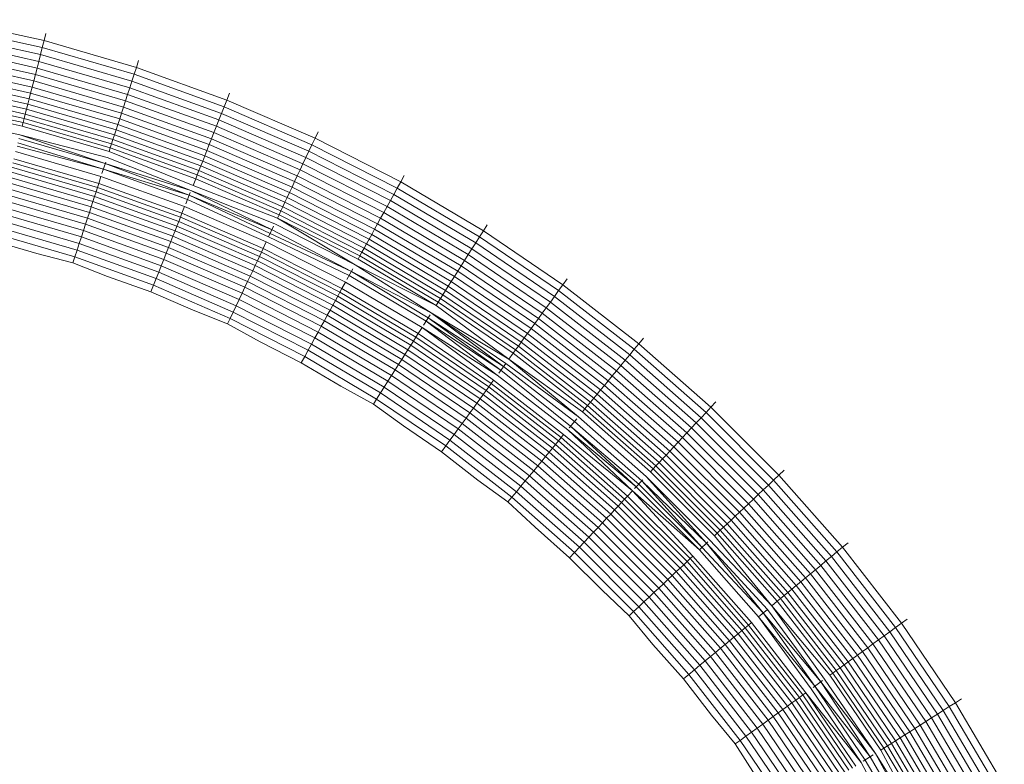
# Model space of a CAD drawing. Units: inches. Extents: x 64 to 1167, y 117 to 939.
# Tile 52 of 56: x 1130.3689 to 1130.6836, y 501.185 to 501.4229. Entities that reach past the tile are written whole.
import ezdxf

# ---------------------------------------------------------------- set-up
doc = ezdxf.new("R2010")
doc.units = ezdxf.units.IN
doc.header["$MEASUREMENT"] = 0
doc.layers.add('A-FLOR-FIXT', color=8, linetype='Continuous', lineweight=18)

msp = doc.modelspace()

# ---------------------------------------------------------------- linework, layer by layer
at = {"layer": 'A-FLOR-FIXT'}
for p, q in [((1130.37673, 501.41624), (1130.34676, 501.42294)), ((1130.37616, 501.41401), (1130.34633, 501.42068)), ((1130.37673, 501.41624), (1130.37731, 501.41848)), ((1130.37504, 501.40963), (1130.34548, 501.41623)), ((1130.3756, 501.41181), (1130.3459, 501.41844)), ((1130.37616, 501.41401), (1130.37673, 501.41624)), ((1130.40623, 501.40767), (1130.37673, 501.41624)), ((1130.37449, 501.40749), (1130.34507, 501.41406)), ((1130.3756, 501.41181), (1130.37616, 501.41401)), ((1130.40552, 501.40549), (1130.37616, 501.41401)), ((1130.37343, 501.40336), (1130.34427, 501.40987)), ((1130.37395, 501.40539), (1130.34466, 501.41194)), ((1130.37449, 501.40749), (1130.37504, 501.40963)), ((1130.37504, 501.40963), (1130.3756, 501.41181)), ((1130.40412, 501.40118), (1130.37504, 501.40963)), ((1130.40481, 501.40332), (1130.3756, 501.41181)), ((1130.40623, 501.40767), (1130.40694, 501.40987)), ((1130.37243, 501.39948), (1130.34352, 501.40595)), ((1130.37292, 501.40138), (1130.34389, 501.40787)), ((1130.37395, 501.40539), (1130.37449, 501.40749)), ((1130.40343, 501.39908), (1130.37449, 501.40749)), ((1130.40552, 501.40549), (1130.40623, 501.40767)), ((1130.43512, 501.39727), (1130.40623, 501.40767)), ((1130.37196, 501.39767), (1130.34317, 501.4041)), ((1130.37292, 501.40138), (1130.37343, 501.40336)), ((1130.37343, 501.40336), (1130.37395, 501.40539)), ((1130.40212, 501.39502), (1130.37343, 501.40336)), ((1130.40277, 501.39702), (1130.37395, 501.40539)), ((1130.40412, 501.40118), (1130.40481, 501.40332)), ((1130.40481, 501.40332), (1130.40552, 501.40549)), ((1130.43344, 501.39301), (1130.40481, 501.40332)), ((1130.43428, 501.39513), (1130.40552, 501.40549)), ((1130.3711, 501.3943), (1130.34252, 501.40069)), ((1130.37152, 501.39594), (1130.34283, 501.40235)), ((1130.37243, 501.39948), (1130.37292, 501.40138)), ((1130.40149, 501.39308), (1130.37292, 501.40138)), ((1130.40343, 501.39908), (1130.40412, 501.40118)), ((1130.43261, 501.39092), (1130.40412, 501.40118)), ((1130.37034, 501.39136), (1130.34195, 501.3977)), ((1130.37071, 501.39278), (1130.34222, 501.39914)), ((1130.37152, 501.39594), (1130.37196, 501.39767)), ((1130.37196, 501.39767), (1130.37243, 501.39948)), ((1130.4003, 501.38943), (1130.37196, 501.39767)), ((1130.40088, 501.39122), (1130.37243, 501.39948)), ((1130.40212, 501.39502), (1130.40277, 501.39702)), ((1130.40277, 501.39702), (1130.40343, 501.39908)), ((1130.431, 501.38686), (1130.40277, 501.39702)), ((1130.4318, 501.38887), (1130.40343, 501.39908)), ((1130.43428, 501.39513), (1130.43512, 501.39727)), ((1130.43512, 501.39727), (1130.43597, 501.39941)), ((1130.46331, 501.38507), (1130.43512, 501.39727)), ((1130.36971, 501.38887), (1130.34147, 501.39518)), ((1130.37001, 501.39005), (1130.34169, 501.39638)), ((1130.37071, 501.39278), (1130.3711, 501.3943)), ((1130.3711, 501.3943), (1130.37152, 501.39594)), ((1130.39923, 501.38613), (1130.3711, 501.3943)), ((1130.39975, 501.38774), (1130.37152, 501.39594)), ((1130.40149, 501.39308), (1130.40212, 501.39502)), ((1130.43023, 501.3849), (1130.40212, 501.39502)), ((1130.43344, 501.39301), (1130.43428, 501.39513)), ((1130.46233, 501.38299), (1130.43428, 501.39513)), ((1130.369, 501.38611), (1130.34093, 501.39238)), ((1130.37001, 501.39005), (1130.37034, 501.39136)), ((1130.37034, 501.39136), (1130.37071, 501.39278)), ((1130.39829, 501.38324), (1130.37034, 501.39136)), ((1130.39874, 501.38463), (1130.37071, 501.39278)), ((1130.4003, 501.38943), (1130.40088, 501.39122)), ((1130.40088, 501.39122), (1130.40149, 501.39308)), ((1130.42876, 501.38118), (1130.40088, 501.39122)), ((1130.42948, 501.38301), (1130.40149, 501.39308)), ((1130.4318, 501.38887), (1130.43261, 501.39092)), ((1130.43261, 501.39092), (1130.43344, 501.39301)), ((1130.4604, 501.37889), (1130.43261, 501.39092)), ((1130.46136, 501.38093), (1130.43344, 501.39301)), ((1130.36971, 501.38887), (1130.37001, 501.39005)), ((1130.3975, 501.3808), (1130.36971, 501.38887)), ((1130.39787, 501.38196), (1130.37001, 501.39005)), ((1130.39923, 501.38613), (1130.39975, 501.38774)), ((1130.39975, 501.38774), (1130.4003, 501.38943)), ((1130.42741, 501.37778), (1130.39975, 501.38774)), ((1130.42806, 501.37944), (1130.4003, 501.38943)), ((1130.431, 501.38686), (1130.4318, 501.38887)), ((1130.45946, 501.37689), (1130.4318, 501.38887)), ((1130.46331, 501.38507), (1130.46429, 501.38716)), ((1130.39624, 501.37695), (1130.3687, 501.38495)), ((1130.39686, 501.37886), (1130.369, 501.38611)), ((1130.39624, 501.37695), (1130.369, 501.38611)), ((1130.39829, 501.38324), (1130.39874, 501.38463)), ((1130.39874, 501.38463), (1130.39923, 501.38613)), ((1130.42621, 501.37474), (1130.39874, 501.38463)), ((1130.42679, 501.37621), (1130.39923, 501.38613)), ((1130.42948, 501.38301), (1130.43023, 501.3849)), ((1130.43023, 501.3849), (1130.431, 501.38686)), ((1130.45765, 501.37304), (1130.43023, 501.3849)), ((1130.45854, 501.37494), (1130.431, 501.38686)), ((1130.46233, 501.38299), (1130.46331, 501.38507)), ((1130.49068, 501.37113), (1130.46331, 501.38507)), ((1130.39491, 501.37284), (1130.36763, 501.38077)), ((1130.39566, 501.37516), (1130.36807, 501.38248)), ((1130.39566, 501.37516), (1130.36836, 501.38364)), ((1130.3975, 501.3808), (1130.39787, 501.38196)), ((1130.42432, 501.36998), (1130.3975, 501.3808)), ((1130.39787, 501.38196), (1130.39829, 501.38324)), ((1130.42517, 501.37213), (1130.39787, 501.38196)), ((1130.42567, 501.37338), (1130.39829, 501.38324)), ((1130.42806, 501.37944), (1130.42876, 501.38118)), ((1130.42876, 501.38118), (1130.42948, 501.38301)), ((1130.45595, 501.36942), (1130.42876, 501.38118)), ((1130.45678, 501.37119), (1130.42948, 501.38301)), ((1130.4604, 501.37889), (1130.46136, 501.38093)), ((1130.46136, 501.38093), (1130.46233, 501.38299)), ((1130.48847, 501.36712), (1130.46136, 501.38093)), ((1130.48957, 501.36911), (1130.46233, 501.38299)), ((1130.3942, 501.37065), (1130.36705, 501.37853)), ((1130.42367, 501.36834), (1130.39686, 501.37886)), ((1130.42679, 501.37621), (1130.42741, 501.37778)), ((1130.42741, 501.37778), (1130.42806, 501.37944)), ((1130.45439, 501.3661), (1130.42741, 501.37778)), ((1130.45515, 501.36772), (1130.42806, 501.37944)), ((1130.45946, 501.37689), (1130.4604, 501.37889)), ((1130.48739, 501.36515), (1130.4604, 501.37889)), ((1130.39333, 501.36797), (1130.36635, 501.37581)), ((1130.39378, 501.36937), (1130.36672, 501.37723)), ((1130.39641, 501.37745), (1130.3952, 501.37375)), ((1130.42254, 501.36548), (1130.39566, 501.37516)), ((1130.42309, 501.36688), (1130.39566, 501.37516)), ((1130.42367, 501.36834), (1130.39624, 501.37695)), ((1130.42309, 501.36688), (1130.39624, 501.37695)), ((1130.42567, 501.37338), (1130.42621, 501.37474)), ((1130.42621, 501.37474), (1130.42679, 501.37621)), ((1130.453, 501.36315), (1130.42621, 501.37474)), ((1130.45367, 501.36458), (1130.42679, 501.37621)), ((1130.45765, 501.37304), (1130.45854, 501.37494)), ((1130.45854, 501.37494), (1130.45946, 501.37689)), ((1130.48528, 501.36131), (1130.45854, 501.37494)), ((1130.48632, 501.36321), (1130.45946, 501.37689)), ((1130.39232, 501.36487), (1130.36554, 501.37265)), ((1130.39284, 501.36647), (1130.36596, 501.37428)), ((1130.39491, 501.37284), (1130.3942, 501.37065)), ((1130.42164, 501.36322), (1130.39491, 501.37284)), ((1130.42432, 501.36998), (1130.42517, 501.37213)), ((1130.42517, 501.37213), (1130.42567, 501.37338)), ((1130.4518, 501.36061), (1130.42517, 501.37213)), ((1130.45237, 501.36182), (1130.42567, 501.37338)), ((1130.45678, 501.37119), (1130.45765, 501.37304)), ((1130.48427, 501.35947), (1130.45765, 501.37304)), ((1130.49068, 501.37113), (1130.49179, 501.37315)), ((1130.39119, 501.36138), (1130.36463, 501.3691)), ((1130.39177, 501.36317), (1130.3651, 501.37092)), ((1130.39378, 501.36937), (1130.39333, 501.36797)), ((1130.3942, 501.37065), (1130.39378, 501.36937)), ((1130.4203, 501.35982), (1130.39378, 501.36937)), ((1130.42079, 501.36107), (1130.3942, 501.37065)), ((1130.45041, 501.35766), (1130.42367, 501.36834)), ((1130.44956, 501.35584), (1130.42367, 501.36834)), ((1130.45128, 501.3595), (1130.42432, 501.36998)), ((1130.45515, 501.36772), (1130.45595, 501.36942)), ((1130.45595, 501.36942), (1130.45678, 501.37119)), ((1130.48234, 501.35597), (1130.45595, 501.36942)), ((1130.48329, 501.35769), (1130.45678, 501.37119)), ((1130.48847, 501.36712), (1130.48957, 501.36911)), ((1130.48957, 501.36911), (1130.49068, 501.37113)), ((1130.51588, 501.35355), (1130.48957, 501.36911)), ((1130.51711, 501.35549), (1130.49068, 501.37113)), ((1130.38995, 501.35758), (1130.36364, 501.36523)), ((1130.39058, 501.35952), (1130.36414, 501.3672)), ((1130.39284, 501.36647), (1130.39232, 501.36487)), ((1130.39333, 501.36797), (1130.39284, 501.36647)), ((1130.41918, 501.35699), (1130.39284, 501.36647)), ((1130.41976, 501.35846), (1130.39333, 501.36797)), ((1130.42342, 501.36772), (1130.42199, 501.3641)), ((1130.44847, 501.35353), (1130.42254, 501.36548)), ((1130.44956, 501.35584), (1130.42309, 501.36688)), ((1130.44898, 501.35461), (1130.42309, 501.36688)), ((1130.45367, 501.36458), (1130.45439, 501.3661)), ((1130.45439, 501.3661), (1130.45515, 501.36772)), ((1130.48058, 501.35276), (1130.45439, 501.3661)), ((1130.48144, 501.35432), (1130.45515, 501.36772)), ((1130.48632, 501.36321), (1130.48739, 501.36515)), ((1130.48739, 501.36515), (1130.48847, 501.36712)), ((1130.51345, 501.34973), (1130.48739, 501.36515)), ((1130.51466, 501.35163), (1130.48847, 501.36712)), ((1130.3893, 501.35558), (1130.36311, 501.36319)), ((1130.39177, 501.36317), (1130.39119, 501.36138)), ((1130.39232, 501.36487), (1130.39177, 501.36317)), ((1130.4179, 501.35376), (1130.39177, 501.36317)), ((1130.41856, 501.35542), (1130.39232, 501.36487)), ((1130.42079, 501.36107), (1130.42164, 501.36322)), ((1130.44772, 501.35193), (1130.42164, 501.36322)), ((1130.45237, 501.36182), (1130.453, 501.36315)), ((1130.453, 501.36315), (1130.45367, 501.36458)), ((1130.47901, 501.3499), (1130.453, 501.36315)), ((1130.47977, 501.35128), (1130.45367, 501.36458)), ((1130.48528, 501.36131), (1130.48632, 501.36321)), ((1130.51227, 501.34786), (1130.48632, 501.36321)), ((1130.38795, 501.35142), (1130.36203, 501.35896)), ((1130.38863, 501.35353), (1130.36258, 501.3611)), ((1130.39058, 501.35952), (1130.38995, 501.35758)), ((1130.39119, 501.36138), (1130.39058, 501.35952)), ((1130.41649, 501.35019), (1130.39058, 501.35952)), ((1130.41721, 501.35202), (1130.39119, 501.36138)), ((1130.41976, 501.35846), (1130.4203, 501.35982)), ((1130.4203, 501.35982), (1130.42079, 501.36107)), ((1130.44616, 501.34863), (1130.4203, 501.35982)), ((1130.44673, 501.34984), (1130.42079, 501.36107)), ((1130.45128, 501.3595), (1130.4518, 501.36061)), ((1130.47608, 501.34458), (1130.45128, 501.3595)), ((1130.47706, 501.34637), (1130.45128, 501.3595)), ((1130.4518, 501.36061), (1130.45237, 501.36182)), ((1130.47765, 501.34744), (1130.4518, 501.36061)), ((1130.4783, 501.34861), (1130.45237, 501.36182)), ((1130.48329, 501.35769), (1130.48427, 501.35947)), ((1130.48427, 501.35947), (1130.48528, 501.36131)), ((1130.50999, 501.34426), (1130.48427, 501.35947)), ((1130.51111, 501.34604), (1130.48528, 501.36131)), ((1130.38726, 501.34929), (1130.36147, 501.35678)), ((1130.3893, 501.35558), (1130.38863, 501.35353)), ((1130.38995, 501.35758), (1130.3893, 501.35558)), ((1130.41496, 501.34634), (1130.3893, 501.35558)), ((1130.41574, 501.3483), (1130.38995, 501.35758)), ((1130.41856, 501.35542), (1130.41918, 501.35699)), ((1130.41918, 501.35699), (1130.41976, 501.35846)), ((1130.44487, 501.34587), (1130.41918, 501.35699)), ((1130.44554, 501.3473), (1130.41976, 501.35846)), ((1130.45006, 501.35692), (1130.44847, 501.35353)), ((1130.47493, 501.34249), (1130.44956, 501.35584)), ((1130.47608, 501.34458), (1130.45041, 501.35766)), ((1130.48144, 501.35432), (1130.48234, 501.35597)), ((1130.48234, 501.35597), (1130.48329, 501.35769)), ((1130.50784, 501.34089), (1130.48234, 501.35597)), ((1130.50889, 501.34254), (1130.48329, 501.35769)), ((1130.51711, 501.35549), (1130.51835, 501.35744)), ((1130.38655, 501.34712), (1130.3609, 501.35457)), ((1130.38863, 501.35353), (1130.38795, 501.35142)), ((1130.41417, 501.34433), (1130.38863, 501.35353)), ((1130.41721, 501.35202), (1130.4179, 501.35376)), ((1130.4179, 501.35376), (1130.41856, 501.35542)), ((1130.44339, 501.34273), (1130.4179, 501.35376)), ((1130.44415, 501.34435), (1130.41856, 501.35542)), ((1130.47421, 501.34117), (1130.44847, 501.35353)), ((1130.47493, 501.34249), (1130.44898, 501.35461)), ((1130.47977, 501.35128), (1130.48058, 501.35276)), ((1130.48058, 501.35276), (1130.48144, 501.35432)), ((1130.50588, 501.33779), (1130.48058, 501.35276)), ((1130.50684, 501.3393), (1130.48144, 501.35432)), ((1130.51466, 501.35163), (1130.51588, 501.35355)), ((1130.51588, 501.35355), (1130.51711, 501.35549)), ((1130.54116, 501.33637), (1130.51588, 501.35355)), ((1130.54251, 501.33823), (1130.51711, 501.35549)), ((1130.37446, 501.34824), (1130.36033, 501.35234)), ((1130.38726, 501.34929), (1130.38655, 501.34712)), ((1130.38795, 501.35142), (1130.38726, 501.34929)), ((1130.41252, 501.34019), (1130.38726, 501.34929)), ((1130.41335, 501.34228), (1130.38795, 501.35142)), ((1130.41574, 501.3483), (1130.41649, 501.35019)), ((1130.41649, 501.35019), (1130.41721, 501.35202)), ((1130.44175, 501.33926), (1130.41649, 501.35019)), ((1130.44259, 501.34103), (1130.41721, 501.35202)), ((1130.44616, 501.34863), (1130.44673, 501.34984)), ((1130.44673, 501.34984), (1130.44772, 501.35193)), ((1130.47192, 501.33701), (1130.44673, 501.34984)), ((1130.47303, 501.33903), (1130.44772, 501.35193)), ((1130.47901, 501.3499), (1130.4783, 501.34861)), ((1130.47977, 501.35128), (1130.47901, 501.3499)), ((1130.50413, 501.33504), (1130.47901, 501.3499)), ((1130.50498, 501.33637), (1130.47977, 501.35128)), ((1130.51227, 501.34786), (1130.51345, 501.34973)), ((1130.51345, 501.34973), (1130.51466, 501.35163)), ((1130.5385, 501.33271), (1130.51345, 501.34973)), ((1130.53982, 501.33453), (1130.51466, 501.35163)), ((1130.38596, 501.34529), (1130.37446, 501.34824)), ((1130.38655, 501.34712), (1130.38596, 501.34529)), ((1130.41169, 501.33807), (1130.38655, 501.34712)), ((1130.41417, 501.34433), (1130.41496, 501.34634)), ((1130.41496, 501.34634), (1130.41574, 501.3483)), ((1130.43999, 501.33551), (1130.41496, 501.34634)), ((1130.44089, 501.33742), (1130.41574, 501.3483)), ((1130.44487, 501.34587), (1130.44554, 501.3473)), ((1130.44554, 501.3473), (1130.44616, 501.34863)), ((1130.47057, 501.33455), (1130.44554, 501.3473)), ((1130.47127, 501.33583), (1130.44616, 501.34863)), ((1130.47765, 501.34744), (1130.47706, 501.34637)), ((1130.50197, 501.33164), (1130.47706, 501.34637)), ((1130.4783, 501.34861), (1130.47765, 501.34744)), ((1130.50263, 501.33267), (1130.47765, 501.34744)), ((1130.50335, 501.3338), (1130.4783, 501.34861)), ((1130.51111, 501.34604), (1130.51227, 501.34786)), ((1130.5372, 501.33092), (1130.51227, 501.34786)), ((1130.397, 501.34092), (1130.38596, 501.34529)), ((1130.41335, 501.34228), (1130.41417, 501.34433)), ((1130.43907, 501.33356), (1130.41417, 501.34433)), ((1130.44339, 501.34273), (1130.44415, 501.34435)), ((1130.44415, 501.34435), (1130.44487, 501.34587)), ((1130.46899, 501.33169), (1130.44415, 501.34435)), ((1130.46981, 501.33316), (1130.44487, 501.34587)), ((1130.47537, 501.34328), (1130.47349, 501.33987)), ((1130.50044, 501.32922), (1130.47608, 501.34458)), ((1130.50197, 501.33164), (1130.47608, 501.34458)), ((1130.50889, 501.34254), (1130.50999, 501.34426)), ((1130.50999, 501.34426), (1130.51111, 501.34604)), ((1130.5347, 501.32747), (1130.50999, 501.34426)), ((1130.53593, 501.32917), (1130.51111, 501.34604)), ((1130.41084, 501.33593), (1130.397, 501.34092)), ((1130.41169, 501.33807), (1130.41252, 501.34019)), ((1130.41252, 501.34019), (1130.41335, 501.34228)), ((1130.43717, 501.32952), (1130.41252, 501.34019)), ((1130.43813, 501.33156), (1130.41335, 501.34228)), ((1130.44175, 501.33926), (1130.44259, 501.34103)), ((1130.44259, 501.34103), (1130.44339, 501.34273)), ((1130.46723, 501.32848), (1130.44259, 501.34103)), ((1130.46813, 501.33012), (1130.44339, 501.34273)), ((1130.49879, 501.32663), (1130.47421, 501.34117)), ((1130.50044, 501.32922), (1130.47493, 501.34249)), ((1130.49948, 501.32771), (1130.47493, 501.34249)), ((1130.50684, 501.3393), (1130.50784, 501.34089)), ((1130.50784, 501.34089), (1130.50889, 501.34254)), ((1130.53235, 501.32423), (1130.50784, 501.34089)), ((1130.5335, 501.32582), (1130.50889, 501.34254)), ((1130.54251, 501.33823), (1130.54387, 501.3401)), ((1130.41084, 501.33593), (1130.41169, 501.33807)), ((1130.4362, 501.32746), (1130.41169, 501.33807)), ((1130.43999, 501.33551), (1130.44089, 501.33742)), ((1130.44089, 501.33742), (1130.44175, 501.33926)), ((1130.4653, 501.32497), (1130.44089, 501.33742)), ((1130.46629, 501.32676), (1130.44175, 501.33926)), ((1130.47192, 501.33701), (1130.47127, 501.33583)), ((1130.47192, 501.33701), (1130.47303, 501.33903)), ((1130.49625, 501.32262), (1130.47192, 501.33701)), ((1130.49749, 501.32457), (1130.47303, 501.33903)), ((1130.50498, 501.33637), (1130.50588, 501.33779)), ((1130.50588, 501.33779), (1130.50684, 501.3393)), ((1130.53019, 501.32127), (1130.50588, 501.33779)), ((1130.53124, 501.32272), (1130.50684, 501.3393)), ((1130.54116, 501.33637), (1130.54251, 501.33823)), ((1130.56678, 501.31941), (1130.54251, 501.33823)), ((1130.42434, 501.33009), (1130.41084, 501.33593)), ((1130.43813, 501.33156), (1130.43907, 501.33356)), ((1130.43907, 501.33356), (1130.43999, 501.33551)), ((1130.46325, 501.32124), (1130.43907, 501.33356)), ((1130.46429, 501.32313), (1130.43999, 501.33551)), ((1130.47057, 501.33455), (1130.46981, 501.33316)), ((1130.47127, 501.33583), (1130.47057, 501.33455)), ((1130.49475, 501.32025), (1130.47057, 501.33455)), ((1130.49553, 501.32149), (1130.47127, 501.33583)), ((1130.50263, 501.33267), (1130.50335, 501.3338)), ((1130.50335, 501.3338), (1130.50413, 501.33504)), ((1130.52741, 501.31745), (1130.50335, 501.3338)), ((1130.50413, 501.33504), (1130.50498, 501.33637)), ((1130.52828, 501.31863), (1130.50413, 501.33504)), ((1130.5292, 501.31991), (1130.50498, 501.33637)), ((1130.5385, 501.33271), (1130.53982, 501.33453)), ((1130.53982, 501.33453), (1130.54116, 501.33637)), ((1130.56387, 501.31588), (1130.53982, 501.33453)), ((1130.56532, 501.31763), (1130.54116, 501.33637)), ((1130.43717, 501.32952), (1130.43813, 501.33156)), ((1130.46218, 501.3193), (1130.43813, 501.33156)), ((1130.46899, 501.33169), (1130.46813, 501.33012)), ((1130.46981, 501.33316), (1130.46899, 501.33169)), ((1130.493, 501.31749), (1130.46899, 501.33169)), ((1130.4939, 501.31892), (1130.46981, 501.33316)), ((1130.50197, 501.33164), (1130.50263, 501.33267)), ((1130.52527, 501.31449), (1130.50197, 501.33164)), ((1130.52662, 501.31636), (1130.50263, 501.33267)), ((1130.53593, 501.32917), (1130.5372, 501.33092)), ((1130.5372, 501.33092), (1130.5385, 501.33271)), ((1130.56102, 501.31244), (1130.5372, 501.33092)), ((1130.56243, 501.31415), (1130.5385, 501.33271)), ((1130.43538, 501.32572), (1130.42434, 501.33009)), ((1130.43538, 501.32572), (1130.4362, 501.32746)), ((1130.4362, 501.32746), (1130.43717, 501.32952)), ((1130.46, 501.31533), (1130.4362, 501.32746)), ((1130.4611, 501.31733), (1130.43717, 501.32952)), ((1130.46723, 501.32848), (1130.46629, 501.32676)), ((1130.46813, 501.33012), (1130.46723, 501.32848)), ((1130.49103, 501.3144), (1130.46723, 501.32848)), ((1130.49204, 501.31599), (1130.46813, 501.33012)), ((1130.50008, 501.32866), (1130.498, 501.32538)), ((1130.52353, 501.31209), (1130.49948, 501.32771)), ((1130.52273, 501.311), (1130.49948, 501.32771)), ((1130.52527, 501.31449), (1130.50044, 501.32922)), ((1130.52423, 501.31306), (1130.50044, 501.32922)), ((1130.52353, 501.31209), (1130.50044, 501.32922)), ((1130.5335, 501.32582), (1130.5347, 501.32747)), ((1130.5347, 501.32747), (1130.53593, 501.32917)), ((1130.5583, 501.30916), (1130.5347, 501.32747)), ((1130.55965, 501.31078), (1130.53593, 501.32917)), ((1130.44579, 501.32), (1130.43538, 501.32572)), ((1130.4653, 501.32497), (1130.46429, 501.32313)), ((1130.46629, 501.32676), (1130.4653, 501.32497)), ((1130.48889, 501.31102), (1130.4653, 501.32497)), ((1130.48998, 501.31274), (1130.46629, 501.32676)), ((1130.49749, 501.32457), (1130.49625, 501.32262)), ((1130.52035, 501.30772), (1130.49749, 501.32457)), ((1130.52155, 501.30937), (1130.49749, 501.32457)), ((1130.52273, 501.311), (1130.49879, 501.32663)), ((1130.52155, 501.30937), (1130.49879, 501.32663)), ((1130.53124, 501.32272), (1130.53235, 501.32423)), ((1130.53235, 501.32423), (1130.5335, 501.32582)), ((1130.55576, 501.30608), (1130.53235, 501.32423)), ((1130.55701, 501.30759), (1130.5335, 501.32582)), ((1130.46325, 501.32124), (1130.46218, 501.3193)), ((1130.46429, 501.32313), (1130.46325, 501.32124)), ((1130.48661, 501.30742), (1130.46325, 501.32124)), ((1130.48777, 501.30925), (1130.46429, 501.32313)), ((1130.49475, 501.32025), (1130.49553, 501.32149)), ((1130.49553, 501.32149), (1130.49625, 501.32262)), ((1130.51884, 501.30564), (1130.49553, 501.32149)), ((1130.51963, 501.30673), (1130.49625, 501.32262)), ((1130.5292, 501.31991), (1130.53019, 501.32127)), ((1130.53019, 501.32127), (1130.53124, 501.32272)), ((1130.55342, 501.30325), (1130.53019, 501.32127)), ((1130.55456, 501.30463), (1130.53124, 501.32272)), ((1130.56678, 501.31941), (1130.56825, 501.32118)), ((1130.4589, 501.31332), (1130.44579, 501.32)), ((1130.46218, 501.3193), (1130.4611, 501.31733)), ((1130.48542, 501.30556), (1130.46218, 501.3193)), ((1130.493, 501.31749), (1130.4939, 501.31892)), ((1130.4939, 501.31892), (1130.49475, 501.32025)), ((1130.51705, 501.30318), (1130.4939, 501.31892)), ((1130.51798, 501.30446), (1130.49475, 501.32025)), ((1130.52741, 501.31745), (1130.52828, 501.31863)), ((1130.52828, 501.31863), (1130.5292, 501.31991)), ((1130.55134, 501.30074), (1130.52828, 501.31863)), ((1130.55235, 501.30196), (1130.5292, 501.31991)), ((1130.56532, 501.31763), (1130.56678, 501.31941)), ((1130.58982, 501.29909), (1130.56678, 501.31941)), ((1130.46, 501.31533), (1130.4589, 501.31332)), ((1130.4611, 501.31733), (1130.46, 501.31533)), ((1130.483, 501.30173), (1130.46, 501.31533)), ((1130.48422, 501.30366), (1130.4611, 501.31733)), ((1130.49103, 501.3144), (1130.49204, 501.31599)), ((1130.49204, 501.31599), (1130.493, 501.31749)), ((1130.51501, 501.30037), (1130.49204, 501.31599)), ((1130.51606, 501.30182), (1130.493, 501.31749)), ((1130.52527, 501.31449), (1130.52662, 501.31636)), ((1130.52662, 501.31636), (1130.52741, 501.31745)), ((1130.54955, 501.29857), (1130.52662, 501.31636)), ((1130.55041, 501.29961), (1130.52741, 501.31745)), ((1130.56243, 501.31415), (1130.56387, 501.31588)), ((1130.56387, 501.31588), (1130.56532, 501.31763)), ((1130.58669, 501.29576), (1130.56387, 501.31588)), ((1130.58825, 501.29742), (1130.56532, 501.31763)), ((1130.47156, 501.30583), (1130.4589, 501.31332)), ((1130.48889, 501.31102), (1130.48998, 501.31274)), ((1130.48998, 501.31274), (1130.49103, 501.3144)), ((1130.51276, 501.29727), (1130.48998, 501.31274)), ((1130.51391, 501.29886), (1130.49103, 501.3144)), ((1130.52423, 501.31306), (1130.52203, 501.31003)), ((1130.54619, 501.29451), (1130.52353, 501.31209)), ((1130.54747, 501.29606), (1130.52423, 501.31306)), ((1130.54877, 501.29763), (1130.52527, 501.31449)), ((1130.54747, 501.29606), (1130.52527, 501.31449)), ((1130.55965, 501.31078), (1130.56102, 501.31244)), ((1130.56102, 501.31244), (1130.56243, 501.31415)), ((1130.58364, 501.29251), (1130.56102, 501.31244)), ((1130.58515, 501.29412), (1130.56243, 501.31415)), ((1130.48661, 501.30742), (1130.48777, 501.30925)), ((1130.48777, 501.30925), (1130.48889, 501.31102)), ((1130.51032, 501.29392), (1130.48777, 501.30925)), ((1130.51156, 501.29562), (1130.48889, 501.31102)), ((1130.54405, 501.29192), (1130.52155, 501.30937)), ((1130.54499, 501.29306), (1130.52273, 501.311)), ((1130.55701, 501.30759), (1130.5583, 501.30916)), ((1130.5583, 501.30916), (1130.55965, 501.31078)), ((1130.58072, 501.2894), (1130.5583, 501.30916)), ((1130.58216, 501.29093), (1130.55965, 501.31078)), ((1130.48197, 501.30011), (1130.47156, 501.30583)), ((1130.48422, 501.30366), (1130.48542, 501.30556)), ((1130.48542, 501.30556), (1130.48661, 501.30742)), ((1130.50775, 501.29038), (1130.48542, 501.30556)), ((1130.50905, 501.29217), (1130.48661, 501.30742)), ((1130.51798, 501.30446), (1130.51884, 501.30564)), ((1130.51884, 501.30564), (1130.51963, 501.30673)), ((1130.54111, 501.28837), (1130.51884, 501.30564)), ((1130.51963, 501.30673), (1130.52035, 501.30772)), ((1130.54197, 501.28941), (1130.51963, 501.30673)), ((1130.54274, 501.29035), (1130.52035, 501.30772)), ((1130.55456, 501.30463), (1130.55576, 501.30608)), ((1130.55576, 501.30608), (1130.55701, 501.30759)), ((1130.57798, 501.28648), (1130.55576, 501.30608)), ((1130.57932, 501.28791), (1130.55701, 501.30759)), ((1130.483, 501.30173), (1130.48422, 501.30366)), ((1130.50643, 501.28856), (1130.48422, 501.30366)), ((1130.51606, 501.30182), (1130.51705, 501.30318)), ((1130.51705, 501.30318), (1130.51798, 501.30446)), ((1130.53917, 501.28603), (1130.51705, 501.30318)), ((1130.54018, 501.28724), (1130.51798, 501.30446)), ((1130.55235, 501.30196), (1130.55342, 501.30325)), ((1130.55342, 501.30325), (1130.55456, 501.30463)), ((1130.57547, 501.28381), (1130.55342, 501.30325)), ((1130.57669, 501.28512), (1130.55456, 501.30463)), ((1130.48197, 501.30011), (1130.483, 501.30173)), ((1130.49157, 501.29313), (1130.48197, 501.30011)), ((1130.50509, 501.28672), (1130.483, 501.30173)), ((1130.51391, 501.29886), (1130.51501, 501.30037)), ((1130.51501, 501.30037), (1130.51606, 501.30182)), ((1130.53696, 501.28335), (1130.51501, 501.30037)), ((1130.53809, 501.28473), (1130.51606, 501.30182)), ((1130.54955, 501.29857), (1130.55041, 501.29961)), ((1130.55041, 501.29961), (1130.55134, 501.30074)), ((1130.57223, 501.28037), (1130.55041, 501.29961)), ((1130.55134, 501.30074), (1130.55235, 501.30196)), ((1130.57324, 501.28143), (1130.55134, 501.30074)), ((1130.57432, 501.28259), (1130.55235, 501.30196)), ((1130.58825, 501.29742), (1130.58982, 501.29909)), ((1130.58982, 501.29909), (1130.5914, 501.30078)), ((1130.61154, 501.27738), (1130.58982, 501.29909)), ((1130.51156, 501.29562), (1130.51276, 501.29727)), ((1130.51276, 501.29727), (1130.51391, 501.29886)), ((1130.53451, 501.28039), (1130.51276, 501.29727)), ((1130.53576, 501.28191), (1130.51391, 501.29886)), ((1130.56908, 501.27701), (1130.54747, 501.29606)), ((1130.54877, 501.29763), (1130.54955, 501.29857)), ((1130.57048, 501.2785), (1130.54877, 501.29763)), ((1130.57131, 501.27939), (1130.54955, 501.29857)), ((1130.58669, 501.29576), (1130.58825, 501.29742)), ((1130.60986, 501.2758), (1130.58825, 501.29742)), ((1130.50374, 501.28486), (1130.49157, 501.29313)), ((1130.50905, 501.29217), (1130.51032, 501.29392)), ((1130.51032, 501.29392), (1130.51156, 501.29562)), ((1130.53187, 501.2772), (1130.51032, 501.29392)), ((1130.53321, 501.27882), (1130.51156, 501.29562)), ((1130.54695, 501.29543), (1130.54456, 501.29255)), ((1130.56596, 501.27369), (1130.54499, 501.29306)), ((1130.56678, 501.27456), (1130.54499, 501.29306)), ((1130.56771, 501.27554), (1130.54619, 501.29451)), ((1130.58364, 501.29251), (1130.58515, 501.29412)), ((1130.58515, 501.29412), (1130.58669, 501.29576)), ((1130.60656, 501.2727), (1130.58515, 501.29412)), ((1130.6082, 501.27424), (1130.58669, 501.29576)), ((1130.50643, 501.28856), (1130.50775, 501.29038)), ((1130.50775, 501.29038), (1130.50905, 501.29217)), ((1130.52908, 501.27384), (1130.50775, 501.29038)), ((1130.53049, 501.27554), (1130.50905, 501.29217)), ((1130.54197, 501.28941), (1130.54274, 501.29035)), ((1130.56475, 501.2724), (1130.54274, 501.29035)), ((1130.56475, 501.2724), (1130.54405, 501.29192)), ((1130.56596, 501.27369), (1130.54405, 501.29192)), ((1130.58072, 501.2894), (1130.58216, 501.29093)), ((1130.58216, 501.29093), (1130.58364, 501.29251)), ((1130.60338, 501.26971), (1130.58216, 501.29093)), ((1130.60495, 501.27119), (1130.58364, 501.29251)), ((1130.50374, 501.28486), (1130.50509, 501.28672)), ((1130.50509, 501.28672), (1130.50643, 501.28856)), ((1130.5262, 501.27035), (1130.50509, 501.28672)), ((1130.52765, 501.2721), (1130.50643, 501.28856)), ((1130.53917, 501.28603), (1130.54018, 501.28724)), ((1130.54018, 501.28724), (1130.54111, 501.28837)), ((1130.56125, 501.26867), (1130.54018, 501.28724)), ((1130.54111, 501.28837), (1130.54197, 501.28941)), ((1130.56225, 501.26973), (1130.54111, 501.28837)), ((1130.56317, 501.27071), (1130.54197, 501.28941)), ((1130.57669, 501.28512), (1130.57798, 501.28648)), ((1130.57798, 501.28648), (1130.57932, 501.28791)), ((1130.59893, 501.26554), (1130.57798, 501.28648)), ((1130.57932, 501.28791), (1130.58072, 501.2894)), ((1130.60036, 501.26688), (1130.57932, 501.28791)), ((1130.60184, 501.26827), (1130.58072, 501.2894)), ((1130.51537, 501.27584), (1130.50374, 501.28486)), ((1130.53576, 501.28191), (1130.53696, 501.28335)), ((1130.53696, 501.28335), (1130.53809, 501.28473)), ((1130.55779, 501.26499), (1130.53696, 501.28335)), ((1130.53809, 501.28473), (1130.53917, 501.28603)), ((1130.55901, 501.26629), (1130.53809, 501.28473)), ((1130.56017, 501.26752), (1130.53917, 501.28603)), ((1130.57432, 501.28259), (1130.57547, 501.28381)), ((1130.57547, 501.28381), (1130.57669, 501.28512)), ((1130.59626, 501.26303), (1130.57547, 501.28381)), ((1130.59756, 501.26425), (1130.57669, 501.28512)), ((1130.53321, 501.27882), (1130.53451, 501.28039)), ((1130.53451, 501.28039), (1130.53576, 501.28191)), ((1130.55516, 501.26219), (1130.53451, 501.28039)), ((1130.5565, 501.26362), (1130.53576, 501.28191)), ((1130.57131, 501.27939), (1130.57223, 501.28037)), ((1130.57223, 501.28037), (1130.57324, 501.28143)), ((1130.59281, 501.25979), (1130.57223, 501.28037)), ((1130.57324, 501.28143), (1130.57432, 501.28259)), ((1130.59388, 501.26079), (1130.57324, 501.28143)), ((1130.59503, 501.26187), (1130.57432, 501.28259)), ((1130.53049, 501.27554), (1130.53187, 501.2772)), ((1130.53187, 501.2772), (1130.53321, 501.27882)), ((1130.55233, 501.25917), (1130.53187, 501.2772)), ((1130.55377, 501.2607), (1130.53321, 501.27882)), ((1130.58837, 501.25562), (1130.56908, 501.27701)), ((1130.58945, 501.25664), (1130.56908, 501.27701)), ((1130.57048, 501.2785), (1130.57131, 501.27939)), ((1130.59094, 501.25803), (1130.57048, 501.2785)), ((1130.59183, 501.25887), (1130.57131, 501.27939)), ((1130.61154, 501.27738), (1130.60986, 501.2758)), ((1130.61322, 501.27896), (1130.61154, 501.27738)), ((1130.63185, 501.25434), (1130.61154, 501.27738)), ((1130.52497, 501.26886), (1130.51537, 501.27584)), ((1130.52765, 501.2721), (1130.52908, 501.27384)), ((1130.52908, 501.27384), (1130.53049, 501.27554)), ((1130.54934, 501.25598), (1130.52908, 501.27384)), ((1130.55085, 501.25759), (1130.53049, 501.27554)), ((1130.56806, 501.27593), (1130.5654, 501.27309)), ((1130.587, 501.25433), (1130.56678, 501.27456)), ((1130.58837, 501.25562), (1130.56771, 501.27554)), ((1130.587, 501.25433), (1130.56771, 501.27554)), ((1130.6082, 501.27424), (1130.60656, 501.2727)), ((1130.60986, 501.2758), (1130.6082, 501.27424)), ((1130.62832, 501.25142), (1130.6082, 501.27424)), ((1130.63008, 501.25287), (1130.60986, 501.2758)), ((1130.5262, 501.27035), (1130.52765, 501.2721)), ((1130.5478, 501.25434), (1130.52765, 501.2721)), ((1130.56225, 501.26973), (1130.56317, 501.27071)), ((1130.56317, 501.27071), (1130.56475, 501.2724)), ((1130.58316, 501.25073), (1130.56317, 501.27071)), ((1130.58405, 501.25156), (1130.56475, 501.2724)), ((1130.58613, 501.25352), (1130.56475, 501.2724)), ((1130.58613, 501.25352), (1130.56596, 501.27369)), ((1130.60495, 501.27119), (1130.60338, 501.26971)), ((1130.60656, 501.2727), (1130.60495, 501.27119)), ((1130.62489, 501.24858), (1130.60495, 501.27119)), ((1130.62659, 501.24999), (1130.60656, 501.2727)), ((1130.52497, 501.26886), (1130.5262, 501.27035)), ((1130.53363, 501.26074), (1130.52497, 501.26886)), ((1130.54624, 501.25268), (1130.5262, 501.27035)), ((1130.55901, 501.26629), (1130.56017, 501.26752)), ((1130.56017, 501.26752), (1130.56125, 501.26867)), ((1130.57996, 501.24772), (1130.56017, 501.26752)), ((1130.56125, 501.26867), (1130.56225, 501.26973)), ((1130.58111, 501.2488), (1130.56125, 501.26867)), ((1130.58218, 501.24981), (1130.56225, 501.26973)), ((1130.60184, 501.26827), (1130.60036, 501.26688)), ((1130.60338, 501.26971), (1130.60184, 501.26827)), ((1130.6216, 501.24586), (1130.60184, 501.26827)), ((1130.62322, 501.2472), (1130.60338, 501.26971)), ((1130.5565, 501.26362), (1130.55779, 501.26499)), ((1130.55779, 501.26499), (1130.55901, 501.26629)), ((1130.57743, 501.24535), (1130.55779, 501.26499)), ((1130.57873, 501.24657), (1130.55901, 501.26629)), ((1130.59893, 501.26554), (1130.59756, 501.26425)), ((1130.60036, 501.26688), (1130.59893, 501.26554)), ((1130.61852, 501.24331), (1130.59893, 501.26554)), ((1130.62003, 501.24456), (1130.60036, 501.26688)), ((1130.55377, 501.2607), (1130.55516, 501.26219)), ((1130.55516, 501.26219), (1130.5565, 501.26362)), ((1130.57463, 501.24272), (1130.55516, 501.26219)), ((1130.57606, 501.24406), (1130.5565, 501.26362)), ((1130.59503, 501.26187), (1130.59388, 501.26079)), ((1130.59626, 501.26303), (1130.59503, 501.26187)), ((1130.6144, 501.2399), (1130.59503, 501.26187)), ((1130.59756, 501.26425), (1130.59626, 501.26303)), ((1130.6157, 501.24098), (1130.59626, 501.26303)), ((1130.61707, 501.24212), (1130.59756, 501.26425)), ((1130.54466, 501.25101), (1130.53363, 501.26074)), ((1130.55085, 501.25759), (1130.55233, 501.25917)), ((1130.55233, 501.25917), (1130.55377, 501.2607)), ((1130.57161, 501.23988), (1130.55233, 501.25917)), ((1130.57315, 501.24132), (1130.55377, 501.2607)), ((1130.59183, 501.25887), (1130.59094, 501.25803)), ((1130.60924, 501.23563), (1130.59094, 501.25803)), ((1130.59281, 501.25979), (1130.59183, 501.25887)), ((1130.61102, 501.23711), (1130.59183, 501.25887)), ((1130.59388, 501.26079), (1130.59281, 501.25979)), ((1130.61205, 501.23796), (1130.59281, 501.25979)), ((1130.61318, 501.2389), (1130.59388, 501.26079)), ((1130.5478, 501.25434), (1130.54934, 501.25598)), ((1130.54934, 501.25598), (1130.55085, 501.25759)), ((1130.56843, 501.23689), (1130.54934, 501.25598)), ((1130.57004, 501.2384), (1130.55085, 501.25759)), ((1130.58886, 501.25608), (1130.58613, 501.25352)), ((1130.60649, 501.23336), (1130.58837, 501.25562)), ((1130.60788, 501.23451), (1130.58837, 501.25562)), ((1130.60924, 501.23563), (1130.58945, 501.25664)), ((1130.63185, 501.25434), (1130.63363, 501.25581)), ((1130.54466, 501.25101), (1130.54624, 501.25268)), ((1130.54624, 501.25268), (1130.5478, 501.25434)), ((1130.56512, 501.23379), (1130.54624, 501.25268)), ((1130.56679, 501.23535), (1130.5478, 501.25434)), ((1130.60499, 501.23212), (1130.58613, 501.25352)), ((1130.60649, 501.23336), (1130.587, 501.25433)), ((1130.62832, 501.25142), (1130.63008, 501.25287)), ((1130.63008, 501.25287), (1130.63185, 501.25434)), ((1130.64881, 501.22872), (1130.63008, 501.25287)), ((1130.65067, 501.23007), (1130.63185, 501.25434)), ((1130.55507, 501.2406), (1130.54466, 501.25101)), ((1130.57996, 501.24772), (1130.58111, 501.2488)), ((1130.58111, 501.2488), (1130.58218, 501.24981)), ((1130.59969, 501.22773), (1130.58111, 501.2488)), ((1130.58218, 501.24981), (1130.58316, 501.25073)), ((1130.60081, 501.22867), (1130.58218, 501.24981)), ((1130.58316, 501.25073), (1130.58405, 501.25156)), ((1130.60185, 501.22952), (1130.58316, 501.25073)), ((1130.60279, 501.2303), (1130.58405, 501.25156)), ((1130.62322, 501.2472), (1130.62489, 501.24858)), ((1130.62489, 501.24858), (1130.62659, 501.24999)), ((1130.64336, 501.22476), (1130.62489, 501.24858)), ((1130.62659, 501.24999), (1130.62832, 501.25142)), ((1130.64515, 501.22606), (1130.62659, 501.24999)), ((1130.64697, 501.22738), (1130.62832, 501.25142)), ((1130.57743, 501.24535), (1130.57873, 501.24657)), ((1130.57873, 501.24657), (1130.57996, 501.24772)), ((1130.59717, 501.22565), (1130.57873, 501.24657)), ((1130.59847, 501.22673), (1130.57996, 501.24772)), ((1130.62003, 501.24456), (1130.6216, 501.24586)), ((1130.6216, 501.24586), (1130.62322, 501.2472)), ((1130.63991, 501.22225), (1130.6216, 501.24586)), ((1130.64161, 501.22349), (1130.62322, 501.2472)), ((1130.57315, 501.24132), (1130.57463, 501.24272)), ((1130.57463, 501.24272), (1130.57606, 501.24406)), ((1130.59284, 501.22207), (1130.57463, 501.24272)), ((1130.57606, 501.24406), (1130.57743, 501.24535)), ((1130.59435, 501.22332), (1130.57606, 501.24406)), ((1130.5958, 501.22451), (1130.57743, 501.24535)), ((1130.61707, 501.24212), (1130.61852, 501.24331)), ((1130.61852, 501.24331), (1130.62003, 501.24456)), ((1130.63668, 501.2199), (1130.61852, 501.24331)), ((1130.63826, 501.22106), (1130.62003, 501.24456)), ((1130.56372, 501.23247), (1130.55507, 501.2406)), ((1130.57004, 501.2384), (1130.57161, 501.23988)), ((1130.57315, 501.24132), (1130.57161, 501.23988)), ((1130.58965, 501.21943), (1130.57161, 501.23988)), ((1130.59127, 501.22077), (1130.57315, 501.24132)), ((1130.61318, 501.2389), (1130.6144, 501.2399)), ((1130.6144, 501.2399), (1130.6157, 501.24098)), ((1130.63235, 501.21676), (1130.6144, 501.2399)), ((1130.6157, 501.24098), (1130.61707, 501.24212)), ((1130.63371, 501.21775), (1130.6157, 501.24098)), ((1130.63516, 501.2188), (1130.61707, 501.24212)), ((1130.56679, 501.23535), (1130.56843, 501.23689)), ((1130.56843, 501.23689), (1130.57004, 501.2384)), ((1130.58628, 501.21664), (1130.56843, 501.23689)), ((1130.58798, 501.21805), (1130.57004, 501.2384)), ((1130.60924, 501.23563), (1130.61102, 501.23711)), ((1130.61102, 501.23711), (1130.61205, 501.23796)), ((1130.6288, 501.21418), (1130.61102, 501.23711)), ((1130.61205, 501.23796), (1130.61318, 501.2389)), ((1130.62989, 501.21497), (1130.61205, 501.23796)), ((1130.63107, 501.21583), (1130.61318, 501.2389)), ((1130.56372, 501.23247), (1130.56512, 501.23379)), ((1130.56512, 501.23379), (1130.56679, 501.23535)), ((1130.58279, 501.21375), (1130.56512, 501.23379)), ((1130.58455, 501.21521), (1130.56679, 501.23535)), ((1130.60788, 501.23451), (1130.60499, 501.23212)), ((1130.62496, 501.21139), (1130.60649, 501.23336)), ((1130.62302, 501.20998), (1130.60649, 501.23336)), ((1130.62496, 501.21139), (1130.60788, 501.23451)), ((1130.62781, 501.21346), (1130.60924, 501.23563)), ((1130.62616, 501.21226), (1130.60924, 501.23563)), ((1130.57129, 501.22333), (1130.56372, 501.23247)), ((1130.60185, 501.22952), (1130.60279, 501.2303)), ((1130.62016, 501.2079), (1130.60279, 501.2303)), ((1130.62302, 501.20998), (1130.60499, 501.23212)), ((1130.62182, 501.2091), (1130.60499, 501.23212)), ((1130.64881, 501.22872), (1130.65067, 501.23007)), ((1130.65067, 501.23007), (1130.65254, 501.23143)), ((1130.66794, 501.20467), (1130.65067, 501.23007)), ((1130.59717, 501.22565), (1130.59847, 501.22673)), ((1130.59847, 501.22673), (1130.59969, 501.22773)), ((1130.61563, 501.20461), (1130.59847, 501.22673)), ((1130.59969, 501.22773), (1130.60081, 501.22867)), ((1130.6169, 501.20554), (1130.59969, 501.22773)), ((1130.60081, 501.22867), (1130.60185, 501.22952)), ((1130.61809, 501.2064), (1130.60081, 501.22867)), ((1130.61918, 501.20719), (1130.60185, 501.22952)), ((1130.64515, 501.22606), (1130.64697, 501.22738)), ((1130.64697, 501.22738), (1130.64881, 501.22872)), ((1130.66407, 501.20222), (1130.64697, 501.22738)), ((1130.666, 501.20344), (1130.64881, 501.22872)), ((1130.59435, 501.22332), (1130.5958, 501.22451)), ((1130.5958, 501.22451), (1130.59717, 501.22565)), ((1130.61282, 501.20257), (1130.5958, 501.22451)), ((1130.61426, 501.20362), (1130.59717, 501.22565)), ((1130.63991, 501.22225), (1130.64161, 501.22349)), ((1130.64161, 501.22349), (1130.64336, 501.22476)), ((1130.65848, 501.19867), (1130.64161, 501.22349)), ((1130.64336, 501.22476), (1130.64515, 501.22606)), ((1130.66031, 501.19983), (1130.64336, 501.22476)), ((1130.66217, 501.20101), (1130.64515, 501.22606)), ((1130.58102, 501.21229), (1130.57129, 501.22333)), ((1130.59127, 501.22077), (1130.58965, 501.21943)), ((1130.59127, 501.22077), (1130.59284, 501.22207)), ((1130.60806, 501.19911), (1130.59127, 501.22077)), ((1130.59284, 501.22207), (1130.59435, 501.22332)), ((1130.60971, 501.20031), (1130.59284, 501.22207)), ((1130.6113, 501.20146), (1130.59435, 501.22332)), ((1130.63668, 501.2199), (1130.63826, 501.22106)), ((1130.63826, 501.22106), (1130.63991, 501.22225)), ((1130.65499, 501.19645), (1130.63826, 501.22106)), ((1130.65671, 501.19754), (1130.63991, 501.22225)), ((1130.58628, 501.21664), (1130.58798, 501.21805)), ((1130.58965, 501.21943), (1130.58798, 501.21805)), ((1130.60461, 501.19661), (1130.58798, 501.21805)), ((1130.60636, 501.19788), (1130.58965, 501.21943)), ((1130.63235, 501.21676), (1130.63371, 501.21775)), ((1130.63371, 501.21775), (1130.63516, 501.2188)), ((1130.65024, 501.19344), (1130.63371, 501.21775)), ((1130.63516, 501.2188), (1130.63668, 501.2199)), ((1130.65175, 501.19439), (1130.63516, 501.2188)), ((1130.65333, 501.1954), (1130.63668, 501.2199)), ((1130.58455, 501.21521), (1130.58279, 501.21375)), ((1130.58455, 501.21521), (1130.58628, 501.21664)), ((1130.60101, 501.19399), (1130.58455, 501.21521)), ((1130.60283, 501.19531), (1130.58628, 501.21664)), ((1130.62781, 501.21346), (1130.6288, 501.21418)), ((1130.6288, 501.21418), (1130.62989, 501.21497)), ((1130.64511, 501.19018), (1130.6288, 501.21418)), ((1130.62989, 501.21497), (1130.63107, 501.21583)), ((1130.64624, 501.1909), (1130.62989, 501.21497)), ((1130.63107, 501.21583), (1130.63235, 501.21676)), ((1130.64748, 501.19169), (1130.63107, 501.21583)), ((1130.64881, 501.19253), (1130.63235, 501.21676)), ((1130.58279, 501.21375), (1130.58102, 501.21229)), ((1130.59004, 501.20066), (1130.58102, 501.21229)), ((1130.59916, 501.19265), (1130.58279, 501.21375)), ((1130.6255, 501.21178), (1130.62247, 501.20958)), ((1130.64066, 501.18736), (1130.62496, 501.21139)), ((1130.64236, 501.18843), (1130.62496, 501.21139)), ((1130.64236, 501.18843), (1130.62616, 501.21226)), ((1130.64408, 501.18953), (1130.62781, 501.21346)), ((1130.61918, 501.20719), (1130.62016, 501.2079)), ((1130.63609, 501.18446), (1130.62016, 501.2079)), ((1130.63782, 501.18556), (1130.62016, 501.2079)), ((1130.63782, 501.18556), (1130.62182, 501.2091)), ((1130.63907, 501.18635), (1130.62302, 501.20998)), ((1130.64066, 501.18736), (1130.62302, 501.20998)), ((1130.61426, 501.20362), (1130.61563, 501.20461)), ((1130.61563, 501.20461), (1130.6169, 501.20554)), ((1130.63136, 501.18146), (1130.61563, 501.20461)), ((1130.6169, 501.20554), (1130.61809, 501.2064)), ((1130.63269, 501.1823), (1130.6169, 501.20554)), ((1130.61809, 501.2064), (1130.61918, 501.20719)), ((1130.63393, 501.18309), (1130.61809, 501.2064)), ((1130.63507, 501.18381), (1130.61918, 501.20719)), ((1130.666, 501.20344), (1130.66794, 501.20467)), ((1130.66794, 501.20467), (1130.66989, 501.20591)), ((1130.68357, 501.17823), (1130.66794, 501.20467)), ((1130.60971, 501.20031), (1130.6113, 501.20146)), ((1130.6113, 501.20146), (1130.61282, 501.20257)), ((1130.62684, 501.17859), (1130.6113, 501.20146)), ((1130.61282, 501.20257), (1130.61426, 501.20362)), ((1130.62843, 501.1796), (1130.61282, 501.20257)), ((1130.62994, 501.18055), (1130.61426, 501.20362)), ((1130.66217, 501.20101), (1130.66407, 501.20222)), ((1130.66407, 501.20222), (1130.666, 501.20344)), ((1130.67956, 501.17603), (1130.66407, 501.20222)), ((1130.68156, 501.17713), (1130.666, 501.20344)), ((1130.59761, 501.19152), (1130.59004, 501.20066)), ((1130.60636, 501.19788), (1130.60806, 501.19911)), ((1130.60806, 501.19911), (1130.60971, 501.20031)), ((1130.62347, 501.17645), (1130.60806, 501.19911)), ((1130.62519, 501.17754), (1130.60971, 501.20031)), ((1130.65671, 501.19754), (1130.65848, 501.19867)), ((1130.65848, 501.19867), (1130.66031, 501.19983)), ((1130.67376, 501.17284), (1130.65848, 501.19867)), ((1130.66031, 501.19983), (1130.66217, 501.20101)), ((1130.67565, 501.17388), (1130.66031, 501.19983)), ((1130.67759, 501.17494), (1130.66217, 501.20101)), ((1130.60101, 501.19399), (1130.60283, 501.19531)), ((1130.60283, 501.19531), (1130.60461, 501.19661)), ((1130.618, 501.17298), (1130.60283, 501.19531)), ((1130.60461, 501.19661), (1130.60636, 501.19788)), ((1130.61987, 501.17416), (1130.60461, 501.19661)), ((1130.62169, 501.17532), (1130.60636, 501.19788)), ((1130.65175, 501.19439), (1130.65333, 501.1954)), ((1130.65333, 501.1954), (1130.65499, 501.19645)), ((1130.66841, 501.1699), (1130.65333, 501.1954)), ((1130.65499, 501.19645), (1130.65671, 501.19754)), ((1130.67013, 501.17084), (1130.65499, 501.19645)), ((1130.67191, 501.17183), (1130.65671, 501.19754)), ((1130.59761, 501.19152), (1130.59916, 501.19265)), ((1130.59916, 501.19265), (1130.60101, 501.19399)), ((1130.61418, 501.17055), (1130.59916, 501.19265)), ((1130.6161, 501.17177), (1130.60101, 501.19399)), ((1130.64748, 501.19169), (1130.64881, 501.19253)), ((1130.64881, 501.19253), (1130.65024, 501.19344)), ((1130.66372, 501.16732), (1130.64881, 501.19253)), ((1130.65024, 501.19344), (1130.65175, 501.19439)), ((1130.6652, 501.16813), (1130.65024, 501.19344)), ((1130.66677, 501.16899), (1130.65175, 501.19439)), ((1130.60397, 501.18149), (1130.59761, 501.19152)), ((1130.64408, 501.18953), (1130.64511, 501.19018)), ((1130.65786, 501.1641), (1130.64408, 501.18953)), ((1130.64511, 501.19018), (1130.64624, 501.1909)), ((1130.65988, 501.16521), (1130.64511, 501.19018)), ((1130.64624, 501.1909), (1130.64748, 501.19169)), ((1130.66106, 501.16586), (1130.64624, 501.1909)), ((1130.66234, 501.16656), (1130.64748, 501.19169)), ((1130.64167, 501.188), (1130.63851, 501.18599)), ((1130.65361, 501.16176), (1130.63907, 501.18635)), ((1130.65526, 501.16267), (1130.64066, 501.18736)), ((1130.65786, 501.1641), (1130.64236, 501.18843)), ((1130.65631, 501.16325), (1130.64236, 501.18843)), ((1130.65148, 501.16059), (1130.63782, 501.18556))]:
    msp.add_line(p, q, dxfattribs=at)

doc.saveas('drawing.dxf')
